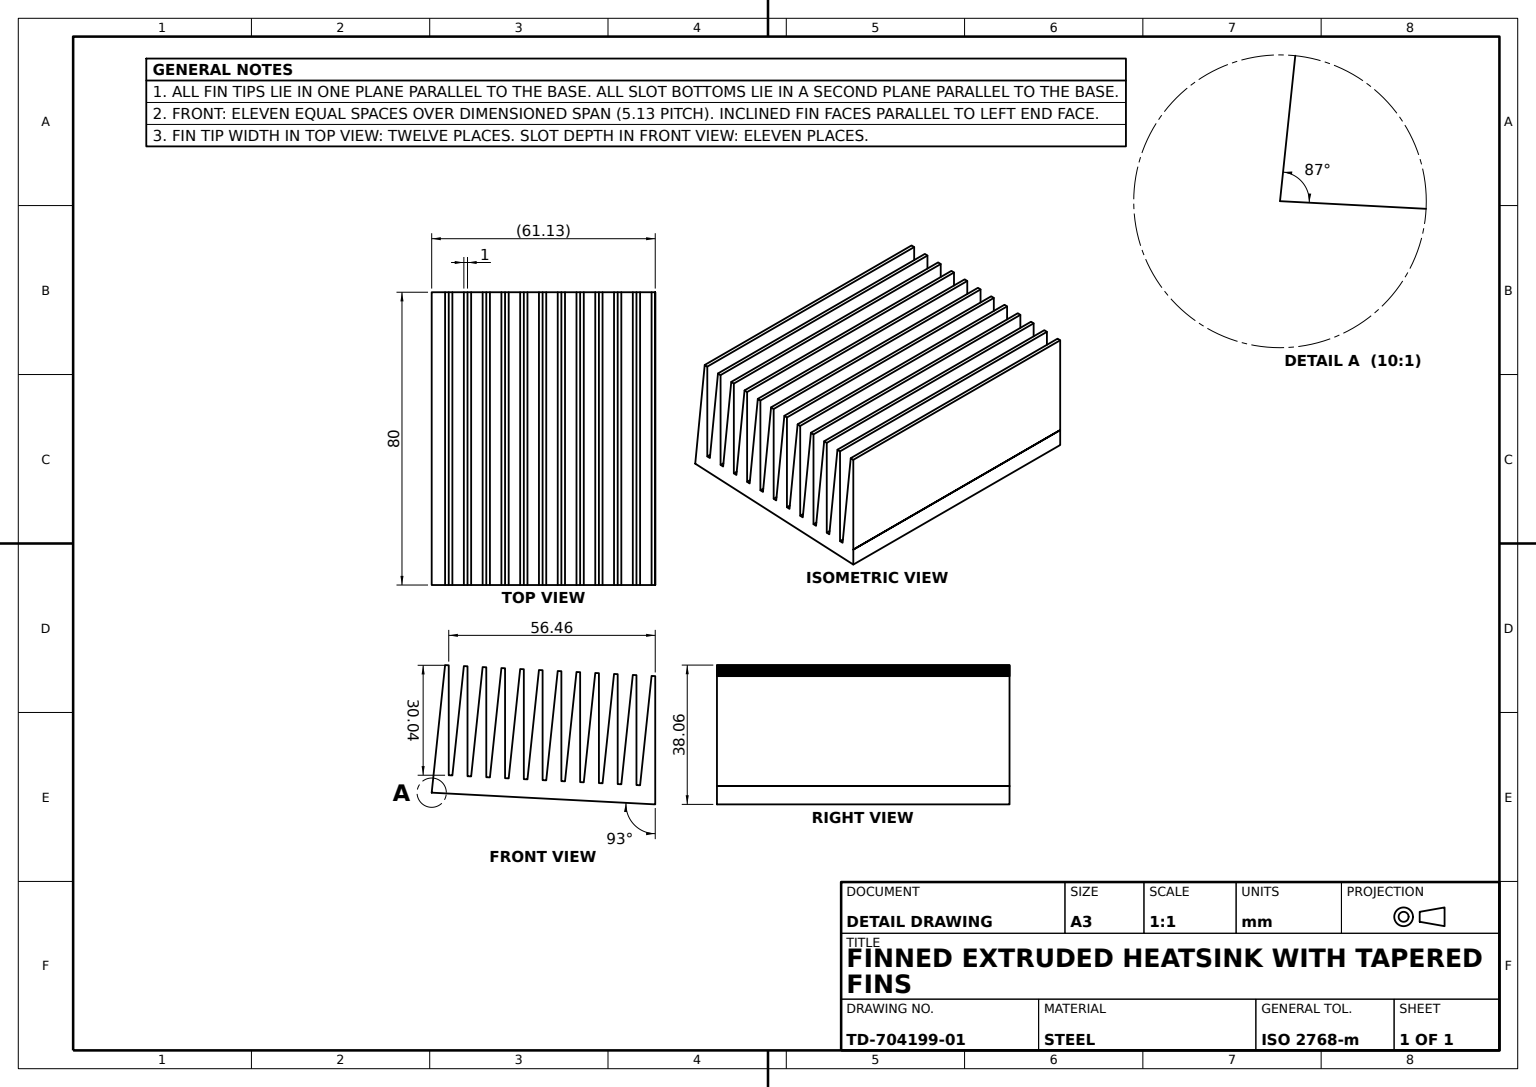
SolidWorks part; units mm, degrees
material "Plain Carbon Steel"
ref_plane "Front Plane" through (0, 0, 0) normal (0, 0, 1) x (1, 0, 0)
ref_plane "Top Plane" through (0, 0, 0) normal (0, 1, 0) x (1, 0, 0)
ref_plane "Right Plane" through (0, 0, 0) normal (1, 0, 0) x (0, 0, -1)
sketch "Base Profile Sketch" plane through (0, 0, 0) normal (0, 1, 0) x (1, 0, 0)
  line L1 (-31.21, -40) -> (30, -40)
  line L2 (-31.21, -40) -> (-31.21, 40)
  line L3 (-31.21, 40) -> (30, 40)
  line L4 (30, -40) -> (30, 40)
  point P0 (0, 0)
  dimension "D1" = 80
  dimension "D2" = 61.21
  dimension "D3" = 30
  dimension "D4" = 40
extrude "Heat Sink Base Block" add sketch "Base Profile Sketch" along normal blind 35
sketch "Fin Slots Sketch" plane through (0, 0, 40) normal (0, 0, 1) x (1, 0, 0)
  line L0 (24.5935, 5) -> (23.0213, 35)
  line L1 (30, 0) -> (59.4133, 0)
  line L2 (30, 0) -> (28.1657, 35)
  line L3 (20.4535, 5) -> (19.458, 5)
  line L4 (-31.21, 35) -> (30, 35) construction
  line L5 (24.5935, 5) -> (25.5935, 5)
  line L6 (22.0257, 35) -> (22.0213, 35)
  line L7 (22.0213, 35) -> (20.449, 5)
  line L8 (-31.21, 0) -> (30, 0) construction
  line L9 (27.1657, 35) -> (25.5935, 5)
  line L10 (27.1657, 35) -> (24.2711, 35)
  line L11 (25.5935, 5) -> (24.5935, 5)
  line L12 (24.598, 5) -> (23.0257, 35)
  line L13 (22.0257, 35) -> (20.4535, 5)
  line L14 (23.0257, 35) -> (23.0213, 35)
  line L15 (19.458, 5) -> (17.8857, 35)
  line L16 (16.8857, 35) -> (15.3135, 5)
  line L17 (23.0213, 35) -> (27.1657, 35)
  line L18 (14.318, 5) -> (12.7457, 35)
  line L19 (11.7457, 35) -> (10.1735, 5)
  line L20 (17.8857, 35) -> (22.0257, 35)
  line L21 (9.178, 5) -> (7.6057, 35)
  line L22 (6.6057, 35) -> (5.0335, 5)
  line L23 (12.7457, 35) -> (16.8857, 35)
  line L24 (4.038, 5) -> (2.4657, 35)
  line L25 (1.4657, 35) -> (-0.1065, 5)
  line L26 (7.6057, 35) -> (11.7457, 35)
  line L27 (-1.102, 5) -> (-2.6743, 35)
  line L28 (-3.6743, 35) -> (-5.2465, 5)
  line L29 (2.4657, 35) -> (6.6057, 35)
  line L30 (-6.242, 5) -> (-7.8143, 35)
  line L31 (-8.8143, 35) -> (-10.3865, 5)
  line L32 (-2.6743, 35) -> (1.4657, 35)
  line L33 (-11.382, 5) -> (-12.9543, 35)
  line L34 (-13.9543, 35) -> (-15.5265, 5)
  line L35 (-7.8143, 35) -> (-3.6743, 35)
  line L36 (-16.522, 5) -> (-18.0943, 35)
  line L37 (-19.0943, 35) -> (-20.6665, 5)
  line L38 (-12.9543, 35) -> (-8.8143, 35)
  line L39 (-21.662, 5) -> (-23.2343, 35)
  line L40 (-24.2343, 35) -> (-25.8065, 5)
  line L41 (-18.0943, 35) -> (-13.9543, 35)
  line L42 (-26.802, 5) -> (-28.3743, 35)
  line L43 (-29.3743, 35) -> (-30.9465, 5)
  line L44 (-23.2343, 35) -> (-19.0943, 35)
  line L45 (-30.9465, 5) -> (-31.2085, 0)
  line L46 (-31.21, 0) -> (-31.2085, 0)
  line L47 (25.5935, 5) -> (24.5935, 5)
  line L48 (15.3135, 5) -> (14.318, 5)
  line L49 (10.1735, 5) -> (9.178, 5)
  line L50 (5.0335, 5) -> (4.038, 5)
  line L51 (-0.1065, 5) -> (-1.102, 5)
  line L52 (-5.2465, 5) -> (-6.242, 5)
  line L53 (-10.3865, 5) -> (-11.382, 5)
  line L54 (-15.5265, 5) -> (-16.522, 5)
  line L55 (-20.6665, 5) -> (-21.662, 5)
  line L56 (-25.8065, 5) -> (-26.802, 5)
  line L57 (-30.9465, 5) -> (-38.008, 5)
  line L58 (-26.802, 5) -> (-26.54, 5)
  line L59 (-31.2085, 0) -> (-31.2085, 35)
  line L60 (-31.2085, 35) -> (-29.3743, 35)
  line L61 (30, 35) -> (30, 0)
  line L62 (30, 35) -> (30, 0) construction
  line L63 (-28.3743, 35) -> (-24.2343, 35)
  line L74 (28.1657, 35) -> (30, 35)
  dimension "D1" = 93
  dimension "D2" = 1
  dimension "D3" = 5
  dimension "D4" = 87
  dimension "D5" = 1
  dimension "D6" = 12
  dimension "D7" = 29.4133
  dimension "D8" = 1.8343
  dimension "D9" = 5.402
  dimension "D11" = 5.7289
  dimension "D54" = 56.54
  dimension "D60" = 61.21
  dimension "D61" = 68.008
extrude "Fin Slots Cut" cut sketch "Fin Slots Sketch" against normal blind 105 contours L59 L57 L43 L42 | L55 L37 L42 L39 | L53 L31 L42 L33 | L52 L28 L42 L30 | L51 L25 L42 L27 | L50 L22 L42 L24 | L12 L11 L9 L42 | L2 L43 L42 | L36 L41 L34 L54 | L21 L26 L19 L49 | L18 L23 L16 L48 | L13 L3 L15 L20
sketch "Side Trim Sketch" plane through (0, 0, 40) normal (0, 0, 1) x (1, 0, 0)
  line L0 (-29.3743, 35) -> (-31.21, 0)
  line L1 (-31.21, 0) -> (-36.7917, 0)
  line L2 (-36.7917, 0) -> (-36.7917, 36.3368)
  line L3 (-36.7917, 36.3368) -> (-29.3743, 36.3368)
  line L4 (-29.3743, 36.3368) -> (-29.3743, 35)
  line L5 (-31.21, 35) -> (-31.21, 0) construction
  line L6 (-31.21, 0) -> (30, 0) construction
  dimension "D1" = 5.5817
  dimension "D2" = 36.3368
extrude "Side Trim Cut" cut sketch "Side Trim Sketch" against normal blind 180.145
